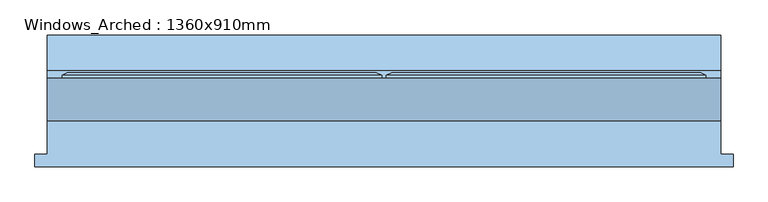
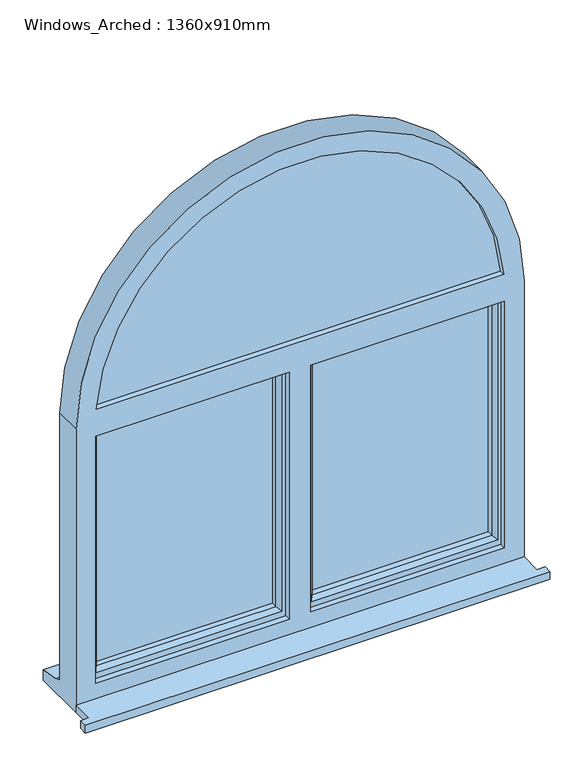
"""IFC4 building model written with IfcOpenShell, lengths in millimetres: window geometry, Windows_Arched : 1360x910mm."""

from ifc_helpers import new_model, si_unit, point, frame, frame_2d, origin, place, context, project, spatial, polyline, circle_curve, trimmed, segment, composite_curve, outline, extrude, faceted_brep, source, transform, mapped, element, save
from ifc_brep_helpers import plane_surface, cylinder_surface, revolved_surface, advanced_brep


def windows_arched_1360x910mm_c5754810(model_context):
    return source(origin(), model_context, "Body", "SolidModel", [
        extrude(outline(polyline([(-990.0, -118.1434322), (-990.0, -93.1434322), (-965.0, -93.1434322), (-965.0, -25.9434322), (395.0, -25.9434322), (395.0, -93.1434322), (420.0, -93.1434322), (420.0, -118.1434322), (-990.0, -118.1434322)])), frame((0.0, 0.0, 1200.0), z_axis=(0.0, 0.0, 1.0), x_axis=(1.0, 0.0, 0.0)), (0.0, 0.0, 1.0), 25.0),
        advanced_brep(
        [(395.0, -25.9434322, 2110.0), (-965.0, -25.9434322, 2110.0), (-965.0, -25.9434322, 1200.0), (395.0, -25.9434322, 1200.0), (-903.5070735, -25.9434322, 2153.0), (333.5070735, -25.9434322, 2153.0), (-905.0, -25.9434322, 1275.0), (-905.0, -25.9434322, 2067.0), (-318.0, -25.9434322, 2067.0), (-318.0, -25.9434322, 1275.0), (335.0, -25.9434322, 1275.0), (-252.0, -25.9434322, 1275.0), (-252.0, -25.9434322, 2067.0), (335.0, -25.9434322, 2067.0), (-965.0, 60.0565678, 2110.0), (-965.0, 60.0565678, 1251.0), (-965.0, 75.0565678, 1250.2709278), (-965.0, 75.0565678, 1246.5550779), (-965.0, 147.5565678, 1233.8088847), (-965.0, 147.5565678, 1200.0), (395.0, 60.0565678, 2110.0), (395.0, 60.0565678, 1251.0), (354.5115323, 60.0565678, 2135.0), (-924.5115323, 60.0565678, 2135.0), (355.0, 60.0565678, 1263.0), (355.0, 60.0565678, 2085.0), (-270.0, 60.0565678, 2085.0), (-270.0, 60.0565678, 1263.0), (-300.0, 60.0565678, 1263.0), (-300.0, 60.0565678, 2085.0), (-925.0, 60.0565678, 2085.0), (-925.0, 60.0565678, 1263.0), (-925.0, -7.9434322, 2085.0), (-925.0, -7.9434322, 1263.0), (355.0, -7.9434322, 1263.0), (-270.0, -7.9434322, 1263.0), (-270.0, -7.9434322, 2085.0), (355.0, -7.9434322, 2085.0), (-252.0, -7.9434322, 1275.0), (335.0, -7.9434322, 1275.0), (335.0, -7.9434322, 2067.0), (-252.0, -7.9434322, 2067.0), (-300.0, -7.9434322, 1263.0), (-300.0, -7.9434322, 2085.0), (-905.0, -7.9434322, 1275.0), (-318.0, -7.9434322, 1275.0), (-318.0, -7.9434322, 2067.0), (-905.0, -7.9434322, 2067.0), (-924.5115323, -7.9434322, 2135.0), (354.5115323, -7.9434322, 2135.0), (333.5070735, -7.9434322, 2153.0), (-903.5070735, -7.9434322, 2153.0), (395.0, 147.5565678, 1200.0), (395.0, 147.5565678, 1233.8088847), (395.0, 75.0565678, 1246.5550779), (395.0, 75.0565678, 1250.2709278)],
        [
            (0, 1, circle_curve(frame((-285.0, -25.9434322, 2110.0), z_axis=(0.0, -1.0, 0.0), x_axis=(-1.0, 0.0, 0.0)), 680.0)),
            (1, 2),
            (2, 3),
            (3, 0),
            (4, 5, circle_curve(frame((-285.0, -25.9434322, 2110.0), z_axis=(0.0, 1.0, 0.0), x_axis=(-1.0, 0.0, 0.0)), 620.0)),
            (5, 4),
            (6, 7),
            (7, 8),
            (8, 9),
            (9, 6),
            (10, 11),
            (11, 12),
            (12, 13),
            (13, 10),
            (1, 14),
            (14, 15),
            (15, 16),
            (16, 17),
            (17, 18),
            (18, 19),
            (19, 2),
            (14, 20, circle_curve(frame((-285.0, 60.0565678, 2110.0), z_axis=(0.0, 1.0, 0.0), x_axis=(-1.0, 0.0, 0.0)), 680.0)),
            (20, 21),
            (21, 15),
            (22, 23, circle_curve(frame((-285.0, 60.0565678, 2110.0), z_axis=(0.0, -1.0, 0.0), x_axis=(-1.0, 0.0, 0.0)), 640.0)),
            (23, 22),
            (24, 25),
            (25, 26),
            (26, 27),
            (27, 24),
            (28, 29),
            (29, 30),
            (30, 31),
            (31, 28),
            (32, 33),
            (33, 31),
            (30, 32),
            (34, 35),
            (35, 36),
            (36, 37),
            (37, 34),
            (38, 39),
            (39, 40),
            (40, 41),
            (41, 38),
            (42, 33),
            (32, 43),
            (43, 42),
            (44, 45),
            (45, 46),
            (46, 47),
            (47, 44),
            (48, 49, circle_curve(frame((-285.0, -7.9434322, 2110.0), z_axis=(0.0, 1.0, 0.0), x_axis=(-1.0, 0.0, 0.0)), 640.0)),
            (49, 48),
            (50, 51, circle_curve(frame((-285.0, -7.9434322, 2110.0), z_axis=(0.0, -1.0, 0.0), x_axis=(-1.0, 0.0, 0.0)), 620.0)),
            (51, 50),
            (6, 44),
            (47, 7),
            (0, 20),
            (48, 23),
            (22, 49),
            (4, 51),
            (50, 5),
            (3, 52),
            (52, 53),
            (53, 54),
            (54, 55),
            (55, 21),
            (24, 34),
            (37, 25),
            (39, 10),
            (13, 40),
            (19, 52),
            (18, 53),
            (17, 54),
            (16, 55),
            (42, 28),
            (27, 35),
            (9, 45),
            (38, 11),
            (43, 29),
            (26, 36),
            (41, 12),
            (8, 46),
        ],
        [
            plane_surface(frame((-905.0, -25.9434322, 1263.0), z_axis=(0.0, -1.0, 0.0), x_axis=(0.0, 0.0, 1.0))),
            plane_surface(frame((-965.0, -25.9434322, 1263.0), z_axis=(-1.0, 0.0, 0.0), x_axis=(0.0, 0.0, 1.0))),
            plane_surface(frame((-965.0, 60.0565678, 1263.0), z_axis=(0.0, 1.0, 0.0), x_axis=(0.0, 0.0, 1.0))),
            plane_surface(frame((-925.0, 60.0565678, 1263.0), z_axis=(1.0, 0.0, 0.0), x_axis=(0.0, 0.0, 1.0))),
            plane_surface(frame((-925.0, -7.9434322, 1263.0), z_axis=(0.0, 1.0, 0.0), x_axis=(0.0, 0.0, 1.0))),
            plane_surface(frame((-905.0, -7.9434322, 1263.0), z_axis=(1.0, 0.0, 0.0), x_axis=(0.0, 0.0, 1.0))),
            cylinder_surface(frame((-285.0, -7.9434322, 2110.0), z_axis=(0.0, 1.0, 0.0), x_axis=(-1.0, 0.0, 0.0)), 680.0),
            revolved_surface(polyline([(-925.0, 60.056567799999996, 2110.0), (-925.0, -7.9434322, 2110.0)]), (-285.0, -7.9434322, 2110.0), (0.0, 1.0, 0.0)),
            revolved_surface(polyline([(-905.0, -7.9434322, 2110.0), (-905.0, -25.9434322, 2110.0)]), (-285.0, -7.9434322, 2110.0), (0.0, 1.0, 0.0)),
            plane_surface(frame((395.0, -25.9434322, 2110.0), z_axis=(1.0, 0.0, 0.0), x_axis=(0.0, 0.0, -1.0))),
            plane_surface(frame((355.0, 60.0565678, 2110.0), z_axis=(-1.0, 0.0, 0.0), x_axis=(0.0, 0.0, -1.0))),
            plane_surface(frame((335.0, -7.9434322, 2110.0), z_axis=(-1.0, 0.0, 0.0), x_axis=(0.0, 0.0, -1.0))),
            plane_surface(frame((395.0, -25.9434322, 1200.0), z_axis=(0.0, 0.0, -1.0), x_axis=(-1.0, 0.0, 0.0))),
            plane_surface(frame((395.0, 147.5565678, 1200.0), z_axis=(0.0, 1.0, 0.0), x_axis=(-1.0, 0.0, 0.0))),
            plane_surface(frame((395.0, 147.5565678, 1233.8088847), z_axis=(0.0, 0.17315391890936818, 0.9848947762915224), x_axis=(-1.0, 0.0, 0.0))),
            plane_surface(frame((395.0, 75.0565678, 1246.5550779), z_axis=(0.0, 1.0, 0.0), x_axis=(-1.0, 0.0, 0.0))),
            plane_surface(frame((395.0, 75.0565678, 1250.2709278), z_axis=(0.0, 0.048547501909150706, 0.998820874861144), x_axis=(-1.0, 0.0, 0.0))),
            plane_surface(frame((395.0, 60.0565678, 1263.0), z_axis=(0.0, 0.0, 1.0), x_axis=(-1.0, 0.0, 0.0))),
            plane_surface(frame((395.0, -7.9434322, 1275.0), z_axis=(0.0, 0.0, 1.0), x_axis=(-1.0, 0.0, 0.0))),
            plane_surface(frame((-300.0, -7.9434322, 1263.0), z_axis=(-1.0, 0.0, 0.0), x_axis=(0.0, 0.0, 1.0))),
            plane_surface(frame((-270.0, 60.0565678, 1263.0), z_axis=(1.0, 0.0, 0.0), x_axis=(0.0, 0.0, 1.0))),
            plane_surface(frame((-252.0, -7.9434322, 1263.0), z_axis=(1.0, 0.0, 0.0), x_axis=(0.0, 0.0, 1.0))),
            plane_surface(frame((-318.0, -25.9434322, 1263.0), z_axis=(-1.0, 0.0, 0.0), x_axis=(0.0, 0.0, 1.0))),
            plane_surface(frame((355.0, -7.9434322, 2085.0), z_axis=(0.0, 0.0, -1.0), x_axis=(-1.0, 0.0, 0.0))),
            plane_surface(frame((355.0, 60.0565678, 2135.0), z_axis=(0.0, 0.0, 1.0), x_axis=(-1.0, 0.0, 0.0))),
            plane_surface(frame((355.0, -7.9434322, 2153.0), z_axis=(0.0, 0.0, 1.0), x_axis=(-1.0, 0.0, 0.0))),
            plane_surface(frame((355.0, -25.9434322, 2067.0), z_axis=(0.0, 0.0, -1.0), x_axis=(-1.0, 0.0, 0.0))),
        ],
        [
            (0, [[1, 2, 3, 4], [5, 6], [7, 8, 9, 10], [11, 12, 13, 14]]),
            (1, [[15, 16, 17, 18, 19, 20, 21, -2]]),
            (2, [[22, 23, 24, -16], [25, 26], [27, 28, 29, 30], [31, 32, 33, 34]]),
            (3, [[35, 36, -33, 37]]),
            (4, [[38, 39, 40, 41], [42, 43, 44, 45]]),
            (4, [[46, -35, 47, 48], [49, 50, 51, 52]]),
            (4, [[53, 54], [55, 56]]),
            (5, [[57, -52, 58, -7]]),
            (6, [[-1, 59, -22, -15]]),
            (7, [[-53, 60, -25, 61]]),
            (8, [[-5, 62, -55, 63]]),
            (9, [[-59, -4, 64, 65, 66, 67, 68, -23]]),
            (10, [[69, -41, 70, -27]]),
            (11, [[71, -14, 72, -43]]),
            (12, [[-64, -3, -21, 73]]),
            (13, [[-65, -73, -20, 74]]),
            (14, [[-66, -74, -19, 75]]),
            (15, [[-67, -75, -18, 76]]),
            (16, [[-68, -76, -17, -24]]),
            (17, [[-36, -46, 77, -34]]),
            (17, [[-69, -30, 78, -38]]),
            (18, [[-57, -10, 79, -49]]),
            (18, [[-71, -42, 80, -11]]),
            (19, [[-31, -77, -48, 81]]),
            (20, [[-29, 82, -39, -78]]),
            (21, [[-80, -45, 83, -12]]),
            (22, [[-79, -9, 84, -50]]),
            (23, [[-32, -81, -47, -37]]),
            (23, [[-40, -82, -28, -70]]),
            (24, [[-26, -60, -54, -61]]),
            (25, [[-6, -63, -56, -62]]),
            (26, [[-13, -83, -44, -72]]),
            (26, [[-51, -84, -8, -58]]),
        ],
    ),
        faceted_brep([(-280.0, 60.0565678, 2095.0), (-280.0, 65.8300705, 2095.0), (-280.0, 65.8300705, 1253.0), (-280.0, 60.0565678, 1253.0), (-270.0, -7.9434322, 2085.0), (-270.0, 60.0565678, 2085.0), (-270.0, 60.0565678, 1263.0), (-270.0, -7.9434322, 1263.0), (-230.0, 6.5494677, 2045.0), (-240.1480377, -7.9434322, 2055.1480377), (-240.1480377, -7.9434322, 1292.8519623), (-230.0, 6.5494677, 1303.0), (-230.0, 24.0565678, 2045.0), (-230.0, 24.0565678, 1303.0), (-240.0, 48.0565678, 2055.0), (-240.0, 24.0565678, 2055.0), (-240.0, 24.0565678, 1293.0), (-240.0, 48.0565678, 1293.0), (-230.0, 65.8300705, 2045.0), (-230.0, 48.0565678, 2045.0), (-230.0, 48.0565678, 1303.0), (-230.0, 65.8300705, 1303.0), (-247.4457548, 71.6035732, 2062.4457548), (-247.4457548, 71.6035732, 1285.5542452), (-269.2153903, 71.6035732, 2084.2153903), (-269.2153903, 71.6035732, 1263.7846097), (365.0, 65.8300705, 1253.0), (365.0, 60.0565678, 1253.0), (355.0, 60.0565678, 1263.0), (355.0, -7.9434322, 1263.0), (325.1480377, -7.9434322, 1292.8519623), (315.0, 6.5494677, 1303.0), (315.0, 24.0565678, 1303.0), (325.0, 24.0565678, 1293.0), (325.0, 48.0565678, 1293.0), (315.0, 48.0565678, 1303.0), (315.0, 65.8300705, 1303.0), (332.4457548, 71.6035732, 1285.5542452), (354.2153903, 71.6035732, 1263.7846097), (365.0, 65.8300705, 2095.0), (365.0, 60.0565678, 2095.0), (355.0, 60.0565678, 2085.0), (355.0, -7.9434322, 2085.0), (325.1480377, -7.9434322, 2055.1480377), (315.0, 6.5494677, 2045.0), (315.0, 24.0565678, 2045.0), (325.0, 24.0565678, 2055.0), (325.0, 48.0565678, 2055.0), (315.0, 48.0565678, 2045.0), (315.0, 65.8300705, 2045.0), (332.4457548, 71.6035732, 2062.4457548), (354.2153903, 71.6035732, 2084.2153903)], [[[0, 1, 2, 3]], [[4, 5, 6, 7]], [[8, 9, 10, 11]], [[12, 8, 11, 13]], [[14, 15, 16, 17]], [[18, 19, 20, 21]], [[22, 18, 21, 23]], [[1, 24, 25, 2]], [[3, 2, 26, 27]], [[7, 6, 28, 29]], [[11, 10, 30, 31]], [[13, 11, 31, 32]], [[17, 16, 33, 34]], [[21, 20, 35, 36]], [[23, 21, 36, 37]], [[2, 25, 38, 26]], [[27, 26, 39, 40]], [[29, 28, 41, 42]], [[31, 30, 43, 44]], [[32, 31, 44, 45]], [[34, 33, 46, 47]], [[36, 35, 48, 49]], [[37, 36, 49, 50]], [[26, 38, 51, 39]], [[40, 39, 1, 0]], [[3, 27, 40, 0], [5, 41, 28, 6]], [[42, 41, 5, 4]], [[7, 29, 42, 4], [9, 43, 30, 10]], [[44, 43, 9, 8]], [[45, 44, 8, 12]], [[15, 46, 33, 16], [13, 32, 45, 12]], [[47, 46, 15, 14]], [[17, 34, 47, 14], [19, 48, 35, 20]], [[49, 48, 19, 18]], [[50, 49, 18, 22]], [[24, 51, 38, 25], [23, 37, 50, 22]], [[39, 51, 24, 1]]]),
        faceted_brep([(-935.0, 60.0565678, 2095.0), (-935.0, 65.8300705, 2095.0), (-935.0, 65.8300705, 1253.0), (-935.0, 60.0565678, 1253.0), (-925.0, -7.9434322, 2085.0), (-925.0, 60.0565678, 2085.0), (-925.0, 60.0565678, 1263.0), (-925.0, -7.9434322, 1263.0), (-885.0, 6.5494677, 2045.0), (-895.1480377, -7.9434322, 2055.1480377), (-895.1480377, -7.9434322, 1292.8519623), (-885.0, 6.5494677, 1303.0), (-885.0, 24.0565678, 2045.0), (-885.0, 24.0565678, 1303.0), (-895.0, 48.0565678, 2055.0), (-895.0, 24.0565678, 2055.0), (-895.0, 24.0565678, 1293.0), (-895.0, 48.0565678, 1293.0), (-885.0, 65.8300705, 2045.0), (-885.0, 48.0565678, 2045.0), (-885.0, 48.0565678, 1303.0), (-885.0, 65.8300705, 1303.0), (-902.4457548, 71.6035732, 2062.4457548), (-902.4457548, 71.6035732, 1285.5542452), (-924.2153903, 71.6035732, 2084.2153903), (-924.2153903, 71.6035732, 1263.7846097), (-290.0, 65.8300705, 1253.0), (-290.0, 60.0565678, 1253.0), (-300.0, 60.0565678, 1263.0), (-300.0, -7.9434322, 1263.0), (-329.8519623, -7.9434322, 1292.8519623), (-340.0, 6.5494677, 1303.0), (-340.0, 24.0565678, 1303.0), (-330.0, 24.0565678, 1293.0), (-330.0, 48.0565678, 1293.0), (-340.0, 48.0565678, 1303.0), (-340.0, 65.8300705, 1303.0), (-322.5542452, 71.6035732, 1285.5542452), (-300.7846097, 71.6035732, 1263.7846097), (-290.0, 65.8300705, 2095.0), (-290.0, 60.0565678, 2095.0), (-300.0, 60.0565678, 2085.0), (-300.0, -7.9434322, 2085.0), (-329.8519623, -7.9434322, 2055.1480377), (-340.0, 6.5494677, 2045.0), (-340.0, 24.0565678, 2045.0), (-330.0, 24.0565678, 2055.0), (-330.0, 48.0565678, 2055.0), (-340.0, 48.0565678, 2045.0), (-340.0, 65.8300705, 2045.0), (-322.5542452, 71.6035732, 2062.4457548), (-300.7846097, 71.6035732, 2084.2153903)], [[[0, 1, 2, 3]], [[4, 5, 6, 7]], [[8, 9, 10, 11]], [[12, 8, 11, 13]], [[14, 15, 16, 17]], [[18, 19, 20, 21]], [[22, 18, 21, 23]], [[1, 24, 25, 2]], [[3, 2, 26, 27]], [[7, 6, 28, 29]], [[11, 10, 30, 31]], [[13, 11, 31, 32]], [[17, 16, 33, 34]], [[21, 20, 35, 36]], [[23, 21, 36, 37]], [[2, 25, 38, 26]], [[27, 26, 39, 40]], [[29, 28, 41, 42]], [[31, 30, 43, 44]], [[32, 31, 44, 45]], [[34, 33, 46, 47]], [[36, 35, 48, 49]], [[37, 36, 49, 50]], [[26, 38, 51, 39]], [[40, 39, 1, 0]], [[3, 27, 40, 0], [5, 41, 28, 6]], [[42, 41, 5, 4]], [[7, 29, 42, 4], [9, 43, 30, 10]], [[44, 43, 9, 8]], [[45, 44, 8, 12]], [[15, 46, 33, 16], [13, 32, 45, 12]], [[47, 46, 15, 14]], [[17, 34, 47, 14], [19, 48, 35, 20]], [[49, 48, 19, 18]], [[50, 49, 18, 22]], [[24, 51, 38, 25], [23, 37, 50, 22]], [[39, 51, 24, 1]]]),
        extrude(outline(polyline([(-330.0, 24.0565678), (-895.0, 24.0565678), (-895.0, 48.0565678), (-330.0, 48.0565678), (-330.0, 24.0565678)])), frame((0.0, 0.0, 1293.0), z_axis=(0.0, 0.0, 1.0), x_axis=(1.0, 0.0, 0.0)), (0.0, 0.0, 1.0), 762.0),
        extrude(outline(polyline([(325.0, 24.0565678), (-240.1480377, 24.0565678), (-240.1480377, 48.0565678), (325.0, 48.0565678), (325.0, 24.0565678)])), frame((0.0, 0.0, 1293.0), z_axis=(0.0, 0.0, 1.0), x_axis=(1.0, 0.0, 0.0)), (0.0, 0.0, 1.0), 762.1480377),
        extrude(outline(composite_curve([segment(polyline([(2135.0, -924.5115323), (2135.0, 354.5115323)]), True, "CONTINUOUS"), segment(trimmed(circle_curve(frame_2d((2110.0, -285.0)), 640.0), [point((2135.0, 354.5115323))], [point((2135.0, -924.5115323))], False, "CARTESIAN"), True, "CONTINUOUS")], self_intersect=False)), frame((0.0, -7.9434322, 0.0), z_axis=(0.0, 1.0, 0.0), x_axis=(0.0, 0.0, 1.0)), (0.0, 0.0, 1.0), 24.0),
        extrude(outline(composite_curve([segment(trimmed(circle_curve(frame_2d((2110.0, -285.0)), 640.0), [point((2135.0, 354.5115323))], [point((2135.0, -924.5115323))], False, "CARTESIAN"), True, "CONTINUOUS"), segment(polyline([(2135.0, -924.5115323), (2135.0, 354.5115323)]), True, "CONTINUOUS")], self_intersect=False), holes=[composite_curve([segment(trimmed(circle_curve(frame_2d((2110.0, -285.0)), 622.0), [point((2153.0, -905.5118855))], [point((2641.0111419, -608.8999338))], True, "CARTESIAN"), True, "CONTINUOUS"), segment(polyline([(2641.0111419, -608.8999338), (2153.0, -327.1465697), (2153.0, -905.5118855)]), True, "CONTINUOUS")], self_intersect=False), composite_curve([segment(polyline([(2153.0, -277.4944465), (2153.0, -292.5055535), (2656.0111419, -582.9191717)]), True, "CONTINUOUS"), segment(trimmed(circle_curve(frame_2d((2110.0, -285.0)), 622.0), [point((2656.0111419, -582.9191717))], [point((2656.0111419, 12.9191717))], True, "CARTESIAN"), True, "CONTINUOUS"), segment(polyline([(2656.0111419, 12.9191717), (2153.0, -277.4944465)]), True, "CONTINUOUS")], self_intersect=False), composite_curve([segment(trimmed(circle_curve(frame_2d((2110.0, -285.0)), 622.0), [point((2641.0111419, 38.8999338))], [point((2153.0, 335.5118855))], True, "CARTESIAN"), True, "CONTINUOUS"), segment(polyline([(2153.0, 335.5118855), (2153.0, -242.8534303), (2641.0111419, 38.8999338)]), True, "CONTINUOUS")], self_intersect=False)]), frame((0.0, 16.0565678, 0.0), z_axis=(0.0, 1.0, 0.0), x_axis=(0.0, 0.0, 1.0)), (0.0, 0.0, 1.0), 39.0),
    ])


if __name__ == "__main__":
    model = new_model("IFC4")
    model_context = context("Model", 3, world=origin())
    ifc_project = project(units=[si_unit("LENGTHUNIT", "METRE", prefix="MILLI")], contexts=[model_context])
    site = spatial("IfcSite", under=ifc_project)
    building = spatial("IfcBuilding", under=site)
    placement = place(None, origin())
    windows_arched_1360x910mm_shape = windows_arched_1360x910mm_c5754810(model_context)
    element("IfcWindow", 1, ObjectType="Windows_Arched : 1360x910mm", at=placement, inside=building, context=model_context, shape_type="MappedRepresentation", body=[
        mapped(windows_arched_1360x910mm_shape, transform((0.0, 0.0, 0.0), x_axis=(1.0, 0.0, 0.0), y_axis=(0.0, 1.0, 0.0), z_axis=(0.0, 0.0, 1.0))),
    ])
    save(model, "model.ifc")

# Revit data of these elements
# Type "Windows_Arched : 1360x910mm"
#   Type Mark = "20"
#   Operation = "UserDefined"
#   Construction Type Id = "GSP4R"
#   Manufacturer = "Revit"
#   Keynote = "L10"
#   Analytic Construction = "1/8 in Pilkington single glazing"
#   Wrap Layers (Ext) from Ext = 0' - 4.03543"
#   Wrap Layers (Int) from Ext = 0' - 6.98819"
#   Window Board Projection = 0' - 0.98425"
#   Window Board Extension = 0' - 0.98425"
#   Visual Light Transmittance = 0.9
#   Solar Heat Gain Coefficient = 0.78
#   Rough Width = 4' - 5.54331"
#   Rough Height = 2' - 11.82677"
#   Height = 2' - 11.82677"
#   Width = 4' - 5.54331"
#   Heat Transfer Coefficient (U) = 0.6496 BTU/(h·ft²·°F)
#   Glazing Thickness = 0' - 0.94488"
#   FrameOffset - External = 0' - 1.9685"
#   Frame Depth = 0' - 2.67717"
#   Default Head Height = 6' - 11.07087"
#   Cill Depth = 0' - 3.44488"
#   Cavity Closer Width = 0' - 1.9685"
#   Cavity Closer Offset from Ext = 0' - 4.03543"
#   Cavity Closer Depth = 0' - 3.34646"
#   Vis - Cavity Closers = yes
#   Define Thermal Properties by = 1
#   Material Trim = Window Frame
#   Material Glass = Glass
#   Material Frame = Window Frame
#   Wall Closure = (empty or 0)
# Element 1 (IfcWindow, "Windows_Arched : 1360x910mm")
#   Materials on its faces: "Window Frame", "Glass"
# Materials
#   "Window Frame": colour RGB 249 249 249, transparency 0
#   "Glass": class "Glass", colour RGB 0 128 192, transparency 0.75, Description = "Soda Lime Glass", Cost = 0
